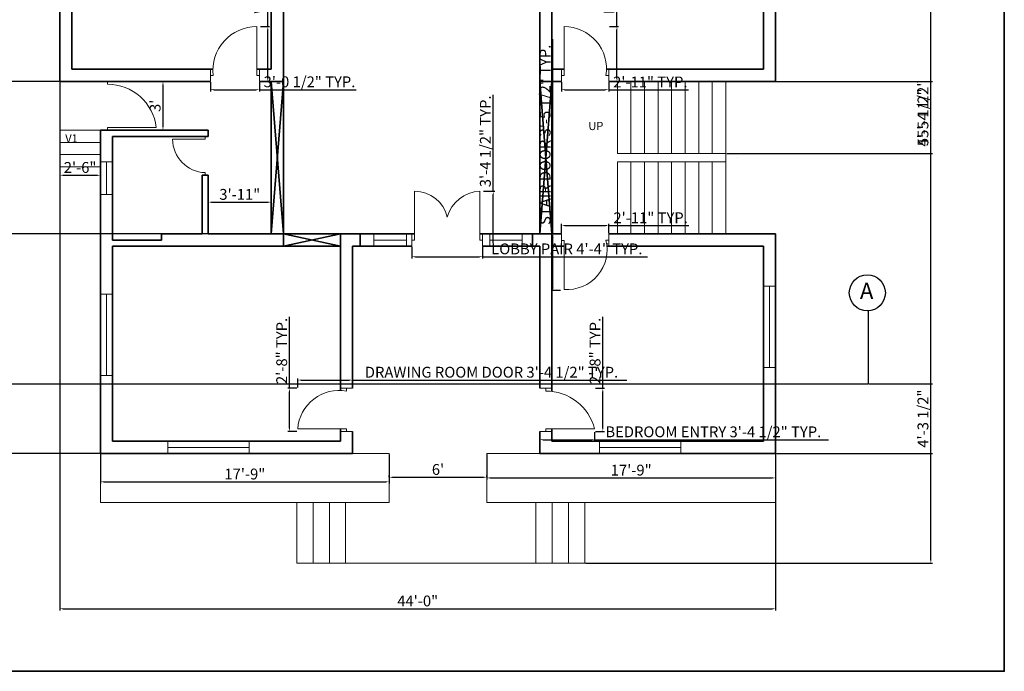
# Model space of a CAD drawing. Units: inches. Extents: x 2257 to 3678, y 834 to 1975.
# Tile 7 of 16: x 2952 to 3678, y 849 to 1330. Entities that reach past the tile are written whole.
import ezdxf

# ---------------------------------------------------------------- set-up
doc = ezdxf.new("R2010")
doc.units = ezdxf.units.IN
for name, color, linetype, lineweight in [('A-ANNO-DIMS', 2, 'Continuous', 18), ('A-ANNO-SYMB', 7, 'Continuous', 25), ('A-ANNO-TEXT', 7, 'Continuous', 18), ('A-ANNO-TTLB', 7, 'Continuous', 35), ('A-DOOR', 3, 'Continuous', 18), ('A-FLOR-STRS', 7, 'Continuous', 18), ('A-GLAZ', 4, 'Continuous', 18), ('A-WALL', 7, 'Continuous', 35)]:
    doc.layers.add(name, color=color, linetype=linetype, lineweight=lineweight)
doc.styles.get("Standard").update_dxf_attribs({"font": 'arial.ttf'})
doc.dimstyles.new('ISO-25', dxfattribs={"dimtxt": 8, "dimasz": 2.5, "dimexe": 1.25, "dimexo": 0.625, "dimtad": 1, "dimdec": 0, "dimlunit": 3, "dimtxsty": 'Standard', "dimcen": 2.5, "dimadec": 0, "dimazin": 0, "dimtfac": 1, "dimtdec": 0, "dimtmove": 0, "dimatfit": 3, "dimfxl": 1, "dimarcsym": 0})

# ---------------------------------------------------------------- blocks, each defined once
blk = doc.blocks.new('*D16')
at = {"layer": 'A-ANNO-DIMS', "color": 0, "lineweight": -2, "transparency": 16777216}
for p, q in [((3051.29, 1284.58), (3058.6, 1284.58)), ((3057.35, 1282.08), (3057.35, 1251.08)), ((3051.29, 1248.58), (3058.6, 1248.58))]:
    blk.add_line(p, q, dxfattribs=at)
at = {"layer": 'A-ANNO-DIMS', "color": 0, "transparency": 16777216}
for points in [[(3056.93, 1282.08), (3057.77, 1282.08), (3057.35, 1284.58)], [(3056.93, 1251.08), (3057.77, 1251.08), (3057.35, 1248.58)]]:
    blk.add_solid(points, dxfattribs=at)
at = {"layer": 'Defpoints', "color": 0, "transparency": 16777216}
for p in [(3050.66, 1284.58), (3050.66, 1248.58), (3057.35, 1248.58)]:
    blk.add_point(p, dxfattribs=at)
at = {"layer": 'A-ANNO-DIMS', "color": 0, "transparency": 16777216, "insert": (3052.64, 1266.58), "char_height": 8, "attachment_point": 5, "rotation": 90}
blk.add_mtext("3'", dxfattribs=at)
blk = doc.blocks.new('*D10')
at = {"layer": 'A-ANNO-DIMS', "color": 0, "lineweight": -2, "transparency": 16777216}
for p, q in [((3090.74, 1196.14), (3090.74, 1196.77)), ((3093.24, 1195.52), (3134.74, 1195.52)), ((3137.24, 1196.14), (3137.24, 1196.77))]:
    blk.add_line(p, q, dxfattribs=at)
at = {"layer": 'A-ANNO-DIMS', "color": 0, "transparency": 16777216}
for points in [[(3093.24, 1195.94), (3093.24, 1195.1), (3090.74, 1195.52)], [(3134.74, 1195.94), (3134.74, 1195.1), (3137.24, 1195.52)]]:
    blk.add_solid(points, dxfattribs=at)
at = {"layer": 'Defpoints', "color": 0, "transparency": 16777216}
for p in [(3090.74, 1195.52), (3137.24, 1195.52), (3137.24, 1195.52)]:
    blk.add_point(p, dxfattribs=at)
at = {"layer": 'A-ANNO-DIMS', "color": 0, "transparency": 16777216, "insert": (3113.99, 1200.23), "char_height": 8, "attachment_point": 5}
blk.add_mtext('3\'-11"', dxfattribs=at)
blk = doc.blocks.new('*D11')
at = {"layer": 'A-ANNO-DIMS', "color": 0, "lineweight": -2, "transparency": 16777216}
for p, q in [((2981.24, 1220.95), (2981.24, 1214.14)), ((3011.24, 1220.95), (3011.24, 1214.14)), ((2983.74, 1215.39), (3008.74, 1215.39))]:
    blk.add_line(p, q, dxfattribs=at)
at = {"layer": 'A-ANNO-DIMS', "color": 0, "transparency": 16777216}
for points in [[(2983.74, 1215.8), (2983.74, 1214.97), (2981.24, 1215.39)], [(3008.74, 1215.8), (3008.74, 1214.97), (3011.24, 1215.39)]]:
    blk.add_solid(points, dxfattribs=at)
at = {"layer": 'Defpoints', "color": 0, "transparency": 16777216}
for p in [(2981.24, 1221.58), (3011.24, 1221.58), (3011.24, 1215.39)]:
    blk.add_point(p, dxfattribs=at)
at = {"layer": 'A-ANNO-DIMS', "color": 0, "transparency": 16777216, "insert": (2996.24, 1220.09), "char_height": 8, "attachment_point": 5}
blk.add_mtext('2\'-6"', dxfattribs=at)
blk = doc.blocks.new('*D12')
at = {"layer": 'A-ANNO-DIMS', "color": 0, "lineweight": -2, "transparency": 16777216}
for p, q in [((3011.24, 1009.45), (3011.24, 987.96)), ((3224.24, 1009.45), (3224.24, 987.96)), ((3013.74, 989.21), (3221.74, 989.21))]:
    blk.add_line(p, q, dxfattribs=at)
at = {"layer": 'A-ANNO-DIMS', "color": 0, "transparency": 16777216}
for points in [[(3013.74, 989.62), (3013.74, 988.79), (3011.24, 989.21)], [(3221.74, 989.62), (3221.74, 988.79), (3224.24, 989.21)]]:
    blk.add_solid(points, dxfattribs=at)
at = {"layer": 'Defpoints', "color": 0, "transparency": 16777216}
for p in [(3011.24, 1010.08), (3224.24, 1010.08), (3224.24, 989.21)]:
    blk.add_point(p, dxfattribs=at)
at = {"layer": 'A-ANNO-DIMS', "color": 0, "transparency": 16777216, "insert": (3117.74, 993.92), "char_height": 8, "attachment_point": 5}
blk.add_mtext('17\'-9"', dxfattribs=at)
blk = doc.blocks.new('*D13')
at = {"layer": 'A-ANNO-DIMS', "color": 0, "lineweight": -2, "transparency": 16777216}
for p, q in [((3296.24, 1009.45), (3296.24, 990.83)), ((3509.24, 1009.45), (3509.24, 990.83)), ((3298.74, 992.08), (3506.74, 992.08))]:
    blk.add_line(p, q, dxfattribs=at)
at = {"layer": 'A-ANNO-DIMS', "color": 0, "transparency": 16777216}
for points in [[(3298.74, 992.49), (3298.74, 991.66), (3296.24, 992.08)], [(3506.74, 992.49), (3506.74, 991.66), (3509.24, 992.08)]]:
    blk.add_solid(points, dxfattribs=at)
at = {"layer": 'Defpoints', "color": 0, "transparency": 16777216}
for p in [(3296.24, 1010.08), (3509.24, 1010.08), (3509.24, 992.08)]:
    blk.add_point(p, dxfattribs=at)
at = {"layer": 'A-ANNO-DIMS', "color": 0, "transparency": 16777216, "insert": (3402.74, 996.79), "char_height": 8, "attachment_point": 5}
blk.add_mtext('17\'-9"', dxfattribs=at)
blk = doc.blocks.new('*D14')
at = {"layer": 'A-ANNO-DIMS', "color": 0, "lineweight": -2, "transparency": 16777216}
for p, q in [((3224.24, 992.7), (3224.24, 993.82)), ((3226.74, 992.57), (3293.74, 992.57)), ((3296.24, 992.7), (3296.24, 993.82))]:
    blk.add_line(p, q, dxfattribs=at)
at = {"layer": 'A-ANNO-DIMS', "color": 0, "transparency": 16777216}
for points in [[(3226.74, 992.99), (3226.74, 992.16), (3224.24, 992.57)], [(3293.74, 992.99), (3293.74, 992.16), (3296.24, 992.57)]]:
    blk.add_solid(points, dxfattribs=at)
at = {"layer": 'Defpoints', "color": 0, "transparency": 16777216}
for p in [(3224.24, 992.08), (3296.24, 992.57), (3296.24, 992.08)]:
    blk.add_point(p, dxfattribs=at)
at = {"layer": 'A-ANNO-DIMS', "color": 0, "transparency": 16777216, "insert": (3260.24, 997.28), "char_height": 8, "attachment_point": 5}
blk.add_mtext("6'", dxfattribs=at)
blk = doc.blocks.new('WIN-60')
for p, q in [((0, 9), (0, 0)), ((60, 4.5), (60, 9)), ((60, 9), (60, 0)), ((0, 0), (0, 4.5)), ((0, 4.5), (60, 4.5))]:
    blk.add_line(p, q)
blk = doc.blocks.new('WIN-60-SIDE')
for p, q in [((0, 60), (9, 60)), ((9, 60), (4.5, 60)), ((4.5, 60), (4.5, 0)), ((9, 0), (0, 0)), ((4.5, 0), (9, 0))]:
    blk.add_line(p, q)
blk = doc.blocks.new('WIN-24')
for p, q in [((0, 9), (0, 0)), ((24, 4.5), (24, 9)), ((24, 9), (24, 0)), ((0, 0), (0, 4.5)), ((0, 4.5), (24, 4.5))]:
    blk.add_line(p, q)
blk = doc.blocks.new('DOOR-WC')
for p, q in [((24, 26.75), (0, 26.75)), ((24, 28.75), (24, 26.75)), ((24, 26.75), (24, 28.75)), ((24, 0), (24, 2)), ((24, 0), (24, 2))]:
    blk.add_line(p, q)
blk.add_arc((24.77, 26.75), 24.77, 180, 268.22548)
blk = doc.blocks.new('DOOR-BEDROOM-WEST')
for p, q in [((34.29, 4.5), (34.29, 40.5)), ((0, 9), (0, 0)), ((36.29, 9), (36.29, 0)), ((0, 0), (0, 4.5)), ((0, 4.5), (2, 4.5)), ((36.29, 4.5), (34.29, 4.5)), ((36.29, 0), (36.29, 4.5)), ((0, 0), (0, 0))]:
    blk.add_line(p, q)
blk.add_arc((34.29, 8.02), 32.48, 90, 186.22352)
blk = doc.blocks.new('DOOR-LOBBY-PAIR')
for p, q in [((2, 4.5), (2, 40.5)), ((50.14, 4.5), (50.14, 40.5)), ((0, 0), (0, 9)), ((0, 9), (0, 4.5)), ((52.14, 9), (52.14, 0)), ((0, 4.5), (2, 4.5)), ((52.14, 4.5), (50.14, 4.5)), ((52.14, 0), (52.14, 4.5))]:
    blk.add_line(p, q)
for centre, radius, start, end in [((2, 15.75), 24.75, 13.39446, 90), ((50.98, 14.71), 25.8, 91.86682, 164.78752)]:
    blk.add_arc(centre, radius, start, end)
blk = doc.blocks.new('DOOR-BEDROOM-EAST')
for p, q in [((2, 4.5), (2, 40.5)), ((0, 9), (0, 0)), ((34.84, 0), (34.84, 9)), ((34.84, 9), (34.84, 4.5)), ((0, 4.5), (2, 4.5)), ((34.84, 4.5), (32.84, 4.5))]:
    blk.add_line(p, q)
blk.add_arc((2, 9.29), 31.21, 351.16993, 90)
blk = doc.blocks.new('DOOR-BEDROOM-FRONT')
for p, q in [((0, 41.01), (0, 32.01)), ((34.84, 36.51), (32.84, 36.51)), ((34.84, 41.01), (34.84, 32.01)), ((34.84, 32.01), (34.84, 36.51)), ((0, 36.08), (2, 36.08)), ((2, 36.08), (2, 0.08))]:
    blk.add_line(p, q)
blk.add_arc((4.15, 29.52), 29.53, 265.82197, 13.68707)
blk = doc.blocks.new('DOOR-DRAWING-ROOM')
for p, q in [((31.5, 31.83), (40.5, 31.83)), ((40.5, 31.83), (36, 31.83)), ((36, 31.83), (36, 29.83)), ((36, 2), (0, 2)), ((36, 0), (36, 2)), ((31.5, 0), (40.5, 0)), ((40.5, 0), (36, 0))]:
    blk.add_line(p, q)
blk.add_arc((30.7, -0.52), 30.81, 80.10035, 175.31629)
blk = doc.blocks.new('DOOR-LOBBY-BEDROOM')
for p, q in [((0, 31.83), (9, 31.83)), ((9, 31.83), (4.5, 31.83)), ((4.5, 31.83), (4.5, 29.83)), ((4.5, 0), (4.5, 2)), ((4.5, 2), (40.5, 2)), ((0, 0), (0, 0)), ((0, 0), (9, 0)), ((9, 0), (4.5, 0))]:
    blk.add_line(p, q)
blk.add_arc((4.5, -7.37), 37.2, 14.58337, 90)
blk = doc.blocks.new('DOOR-SIDE-ENTRY')
for p, q in [((0, 36), (0, 34)), ((0, 0), (0, 2)), ((0, 2), (24, 2)), ((24, 2), (36, 2))]:
    blk.add_line(p, q)
blk.add_arc((0, -2.25), 36.25, 6.73292, 90)
blk = doc.blocks.new('STEPS-VERANDAH')
for p, q in [((0, 80.97), (213, 80.97)), ((0, 44.97), (0, 80.97)), ((0, 80.97), (0, 80.97)), ((213, 80.97), (213, 44.97)), ((213, 80.97), (213, 44.97)), ((498, 80.97), (285, 80.97)), ((285, 80.97), (285, 44.97)), ((285, 80.97), (285, 44.97)), ((498, 44.97), (498, 80.97)), ((213, 44.97), (0, 44.97)), ((144.84, 0), (144.84, 44.97)), ((168.84, 44.97), (156.84, 44.97)), ((156.84, 44.97), (156.84, 0)), ((168.84, 0), (168.84, 44.97)), ((168.84, 44.97), (168.84, 44.97)), ((180.84, 44.97), (180.84, 0)), ((285, 44.97), (498, 44.97)), ((333.2, 44.97), (321.2, 44.97)), ((321.2, 44.97), (321.2, 0)), ((333.2, 0), (333.2, 44.97)), ((357.2, 44.97), (345.2, 44.97)), ((345.2, 44.97), (345.2, 0)), ((357.2, 0), (357.2, 44.97)), ((213, 0), (144.84, 0)), ((156.84, 0), (144.84, 0)), ((180.84, 0), (168.84, 0)), ((213, 0), (357.2, 0)), ((345.2, 0), (333.2, 0))]:
    blk.add_line(p, q)
blk = doc.blocks.new('STEPS-SIDE-ENTRY')
for p, q in [((0, 69.18), (0, 3.09)), ((30, 30.09), (0, 30.09)), ((30, 18), (30, 27)), ((0, 12.09), (0, 21.09)), ((0, 21.09), (30, 21.09)), ((30, 12.09), (0, 12.09)), ((30, 0), (30, 9)), ((0, 3.09), (30, 3.09))]:
    blk.add_line(p, q)
blk = doc.blocks.new('*D64')
at = {"layer": 'A-ANNO-DIMS', "color": 0, "lineweight": -2, "transparency": 16777216}
for p, q in [((3134.67, 1325.08), (3134.67, 1529.43)), ((3129.22, 1325.08), (3135.92, 1325.08)), ((3134.67, 1287.08), (3134.67, 1322.58)), ((3129.22, 1284.58), (3135.92, 1284.58))]:
    blk.add_line(p, q, dxfattribs=at)
at = {"layer": 'A-ANNO-DIMS', "color": 0, "transparency": 16777216}
for points in [[(3134.25, 1322.58), (3135.09, 1322.58), (3134.67, 1325.08)], [(3134.25, 1287.08), (3135.09, 1287.08), (3134.67, 1284.58)]]:
    blk.add_solid(points, dxfattribs=at)
at = {"layer": 'Defpoints', "color": 0, "transparency": 16777216}
for p in [(3128.6, 1325.08), (3134.67, 1325.08), (3128.6, 1284.58)]:
    blk.add_point(p, dxfattribs=at)
at = {"layer": 'A-ANNO-DIMS', "color": 0, "transparency": 16777216, "insert": (3129.9, 1428.5), "char_height": 8, "attachment_point": 5, "rotation": 90}
blk.add_mtext('WEST BEDROOM DOOR 3\'-4 1/2" TYP.', dxfattribs=at)
blk = doc.blocks.new('*D65')
at = {"layer": 'A-ANNO-DIMS', "color": 0, "lineweight": -2, "transparency": 16777216}
for p, q in [((3092.31, 1283.95), (3092.31, 1277.25)), ((3094.81, 1278.5), (3126.1, 1278.5)), ((3128.6, 1283.95), (3128.6, 1277.25)), ((3128.6, 1278.5), (3199.75, 1278.5))]:
    blk.add_line(p, q, dxfattribs=at)
at = {"layer": 'A-ANNO-DIMS', "color": 0, "transparency": 16777216}
for points in [[(3094.81, 1278.92), (3094.81, 1278.09), (3092.31, 1278.5)], [(3126.1, 1278.92), (3126.1, 1278.09), (3128.6, 1278.5)]]:
    blk.add_solid(points, dxfattribs=at)
at = {"layer": 'Defpoints', "color": 0, "transparency": 16777216}
for p in [(3092.31, 1284.58), (3128.6, 1284.58), (3128.6, 1278.5)]:
    blk.add_point(p, dxfattribs=at)
at = {"layer": 'A-ANNO-DIMS', "color": 0, "transparency": 16777216, "insert": (3165.42, 1283.27), "char_height": 8, "attachment_point": 5}
blk.add_mtext('3\'-0 1/2" TYP.', dxfattribs=at)
blk = doc.blocks.new('*D66')
at = {"layer": 'A-ANNO-DIMS', "color": 0, "lineweight": -2, "transparency": 16777216}
for p, q in [((3392.2, 1325.08), (3392.2, 1525.59)), ((3386.75, 1325.08), (3393.45, 1325.08)), ((3392.2, 1287.08), (3392.2, 1322.58)), ((3386.75, 1284.58), (3393.45, 1284.58))]:
    blk.add_line(p, q, dxfattribs=at)
at = {"layer": 'A-ANNO-DIMS', "color": 0, "transparency": 16777216}
for points in [[(3391.79, 1322.58), (3392.62, 1322.58), (3392.2, 1325.08)], [(3391.79, 1287.08), (3392.62, 1287.08), (3392.2, 1284.58)]]:
    blk.add_solid(points, dxfattribs=at)
at = {"layer": 'Defpoints', "color": 0, "transparency": 16777216}
for p in [(3386.13, 1325.08), (3392.2, 1325.08), (3386.13, 1284.58)]:
    blk.add_point(p, dxfattribs=at)
at = {"layer": 'A-ANNO-DIMS', "color": 0, "transparency": 16777216, "insert": (3387.44, 1426.58), "char_height": 8, "attachment_point": 5, "rotation": 90}
blk.add_mtext('EAST BEDROOM DOOR 3\'-4 1/2" TYP.', dxfattribs=at)
blk = doc.blocks.new('*D67')
at = {"layer": 'A-ANNO-DIMS', "color": 0, "lineweight": -2, "transparency": 16777216}
for p, q in [((3351.29, 1283.95), (3351.29, 1277.25)), ((3353.79, 1278.5), (3383.63, 1278.5)), ((3386.13, 1283.95), (3386.13, 1277.25)), ((3386.13, 1278.5), (3445, 1278.5))]:
    blk.add_line(p, q, dxfattribs=at)
at = {"layer": 'A-ANNO-DIMS', "color": 0, "transparency": 16777216}
for points in [[(3353.79, 1278.92), (3353.79, 1278.09), (3351.29, 1278.5)], [(3383.63, 1278.92), (3383.63, 1278.09), (3386.13, 1278.5)]]:
    blk.add_solid(points, dxfattribs=at)
at = {"layer": 'Defpoints', "color": 0, "transparency": 16777216}
for p in [(3351.29, 1284.58), (3386.13, 1284.58), (3386.13, 1278.5)]:
    blk.add_point(p, dxfattribs=at)
at = {"layer": 'A-ANNO-DIMS', "color": 0, "transparency": 16777216, "insert": (3416.81, 1283.15), "char_height": 8, "attachment_point": 5}
blk.add_mtext('2\'-11" TYP.', dxfattribs=at)
blk = doc.blocks.new('*D68')
at = {"layer": 'A-ANNO-DIMS', "color": 0, "lineweight": -2, "transparency": 16777216}
for p, q in [((3345.05, 1172.08), (3345.05, 1315.84)), ((3350.66, 1172.08), (3343.8, 1172.08)), ((3345.05, 1132.95), (3345.05, 1169.58)), ((3350.66, 1130.45), (3343.8, 1130.45))]:
    blk.add_line(p, q, dxfattribs=at)
at = {"layer": 'A-ANNO-DIMS', "color": 0, "transparency": 16777216}
for points in [[(3344.63, 1169.58), (3345.46, 1169.58), (3345.05, 1172.08)], [(3344.63, 1132.95), (3345.46, 1132.95), (3345.05, 1130.45)]]:
    blk.add_solid(points, dxfattribs=at)
at = {"layer": 'Defpoints', "color": 0, "transparency": 16777216}
for p in [(3345.05, 1172.08), (3351.29, 1172.08), (3351.29, 1130.45)]:
    blk.add_point(p, dxfattribs=at)
at = {"layer": 'A-ANNO-DIMS', "color": 0, "transparency": 16777216, "insert": (3340.28, 1245.21), "char_height": 8, "attachment_point": 5, "rotation": 90}
blk.add_mtext('STAIR DOOR 3\'-5 1/2" TYP.', dxfattribs=at)
blk = doc.blocks.new('*D69')
at = {"layer": 'A-ANNO-DIMS', "color": 0, "lineweight": -2, "transparency": 16777216}
for p, q in [((3351.29, 1172.7), (3351.29, 1179.57)), ((3353.79, 1178.32), (3383.86, 1178.32)), ((3386.36, 1172.7), (3386.36, 1179.57)), ((3386.36, 1178.32), (3445.23, 1178.32))]:
    blk.add_line(p, q, dxfattribs=at)
at = {"layer": 'A-ANNO-DIMS', "color": 0, "transparency": 16777216}
for points in [[(3353.79, 1178.74), (3353.79, 1177.9), (3351.29, 1178.32)], [(3383.86, 1178.74), (3383.86, 1177.9), (3386.36, 1178.32)]]:
    blk.add_solid(points, dxfattribs=at)
at = {"layer": 'Defpoints', "color": 0, "transparency": 16777216}
for p in [(3386.36, 1178.32), (3351.29, 1172.08), (3386.36, 1172.08)]:
    blk.add_point(p, dxfattribs=at)
at = {"layer": 'A-ANNO-DIMS', "color": 0, "transparency": 16777216, "insert": (3417.05, 1182.96), "char_height": 8, "attachment_point": 5}
blk.add_mtext('2\'-11" TYP.', dxfattribs=at)
blk = doc.blocks.new('*D74')
at = {"layer": 'A-ANNO-DIMS', "color": 0, "lineweight": -2, "transparency": 16777216}
for p, q in [((3241.01, 1162.45), (3241.01, 1154.01)), ((3293.15, 1162.45), (3293.15, 1154.01)), ((3243.51, 1155.26), (3290.65, 1155.26)), ((3293.15, 1155.26), (3414.87, 1155.26))]:
    blk.add_line(p, q, dxfattribs=at)
at = {"layer": 'A-ANNO-DIMS', "color": 0, "transparency": 16777216}
for points in [[(3243.51, 1155.67), (3243.51, 1154.84), (3241.01, 1155.26)], [(3290.65, 1155.67), (3290.65, 1154.84), (3293.15, 1155.26)]]:
    blk.add_solid(points, dxfattribs=at)
at = {"layer": 'Defpoints', "color": 0, "transparency": 16777216}
for p in [(3241.01, 1163.08), (3293.15, 1163.08), (3293.15, 1155.26)]:
    blk.add_point(p, dxfattribs=at)
at = {"layer": 'A-ANNO-DIMS', "color": 0, "transparency": 16777216, "insert": (3355.26, 1160.02), "char_height": 8, "attachment_point": 5}
blk.add_mtext('LOBBY PAIR 4\'-4" TYP.', dxfattribs=at)
blk = doc.blocks.new('*D75')
at = {"layer": 'A-ANNO-DIMS', "color": 0, "lineweight": -2, "transparency": 16777216}
for p, q in [((3300.97, 1203.58), (3300.97, 1274.73)), ((3293.77, 1203.58), (3302.22, 1203.58)), ((3300.97, 1165.58), (3300.97, 1201.08)), ((3293.77, 1163.08), (3302.22, 1163.08))]:
    blk.add_line(p, q, dxfattribs=at)
at = {"layer": 'A-ANNO-DIMS', "color": 0, "transparency": 16777216}
for points in [[(3300.55, 1201.08), (3301.38, 1201.08), (3300.97, 1203.58)], [(3300.55, 1165.58), (3301.38, 1165.58), (3300.97, 1163.08)]]:
    blk.add_solid(points, dxfattribs=at)
at = {"layer": 'Defpoints', "color": 0, "transparency": 16777216}
for p in [(3293.15, 1203.58), (3300.97, 1203.58), (3293.15, 1163.08)]:
    blk.add_point(p, dxfattribs=at)
at = {"layer": 'A-ANNO-DIMS', "color": 0, "transparency": 16777216, "insert": (3296.2, 1240.4), "char_height": 8, "attachment_point": 5, "rotation": 90}
blk.add_mtext('3\'-4 1/2" TYP.', dxfattribs=at)
blk = doc.blocks.new('*D76')
at = {"layer": 'A-ANNO-DIMS', "color": 0, "lineweight": -2, "transparency": 16777216}
for p, q in [((3156.74, 1058.81), (3156.74, 1065.51)), ((3159.24, 1064.26), (3194.74, 1064.26)), ((3197.24, 1058.81), (3197.24, 1065.51)), ((3197.24, 1064.26), (3399.62, 1064.26))]:
    blk.add_line(p, q, dxfattribs=at)
at = {"layer": 'A-ANNO-DIMS', "color": 0, "transparency": 16777216}
for points in [[(3159.24, 1064.68), (3159.24, 1063.85), (3156.74, 1064.26)], [(3194.74, 1064.68), (3194.74, 1063.85), (3197.24, 1064.26)]]:
    blk.add_solid(points, dxfattribs=at)
at = {"layer": 'Defpoints', "color": 0, "transparency": 16777216}
for p in [(3197.24, 1064.26), (3156.74, 1058.19), (3197.24, 1058.19)]:
    blk.add_point(p, dxfattribs=at)
at = {"layer": 'A-ANNO-DIMS', "color": 0, "transparency": 16777216, "insert": (3299.68, 1069.03), "char_height": 8, "attachment_point": 5}
blk.add_mtext('DRAWING ROOM DOOR 3\'-4 1/2" TYP.', dxfattribs=at)
blk = doc.blocks.new('*D77')
at = {"layer": 'A-ANNO-DIMS', "color": 0, "lineweight": -2, "transparency": 16777216}
for p, q in [((3150.67, 1058.19), (3150.67, 1110.84)), ((3156.12, 1058.19), (3149.42, 1058.19)), ((3150.67, 1028.85), (3150.67, 1055.69)), ((3156.12, 1026.35), (3149.42, 1026.35))]:
    blk.add_line(p, q, dxfattribs=at)
at = {"layer": 'A-ANNO-DIMS', "color": 0, "transparency": 16777216}
for points in [[(3150.25, 1055.69), (3151.08, 1055.69), (3150.67, 1058.19)], [(3150.25, 1028.85), (3151.08, 1028.85), (3150.67, 1026.35)]]:
    blk.add_solid(points, dxfattribs=at)
at = {"layer": 'Defpoints', "color": 0, "transparency": 16777216}
for p in [(3150.67, 1058.19), (3156.74, 1058.19), (3156.74, 1026.35)]:
    blk.add_point(p, dxfattribs=at)
at = {"layer": 'A-ANNO-DIMS', "color": 0, "transparency": 16777216, "insert": (3145.96, 1085.76), "char_height": 8, "attachment_point": 5, "rotation": 90}
blk.add_mtext('2\'-8" TYP.', dxfattribs=at)
blk = doc.blocks.new('*D78')
at = {"layer": 'A-ANNO-DIMS', "color": 0, "lineweight": -2, "transparency": 16777216}
for p, q in [((3335.24, 1025.73), (3335.24, 1019.03)), ((3375.74, 1025.73), (3375.74, 1019.03)), ((3337.74, 1020.28), (3373.24, 1020.28)), ((3375.74, 1020.28), (3548.37, 1020.28))]:
    blk.add_line(p, q, dxfattribs=at)
at = {"layer": 'A-ANNO-DIMS', "color": 0, "transparency": 16777216}
for points in [[(3337.74, 1020.7), (3337.74, 1019.86), (3335.24, 1020.28)], [(3373.24, 1020.7), (3373.24, 1019.86), (3375.74, 1020.28)]]:
    blk.add_solid(points, dxfattribs=at)
at = {"layer": 'Defpoints', "color": 0, "transparency": 16777216}
for p in [(3335.24, 1026.35), (3375.74, 1026.35), (3375.74, 1020.28)]:
    blk.add_point(p, dxfattribs=at)
at = {"layer": 'A-ANNO-DIMS', "color": 0, "transparency": 16777216, "insert": (3463.31, 1025.05), "char_height": 8, "attachment_point": 5}
blk.add_mtext('BEDROOM ENTRY 3\'-4 1/2" TYP.', dxfattribs=at)
blk = doc.blocks.new('*D79')
at = {"layer": 'A-ANNO-DIMS', "color": 0, "lineweight": -2, "transparency": 16777216}
for p, q in [((3381.82, 1058.19), (3381.82, 1110.84)), ((3376.37, 1058.19), (3383.07, 1058.19)), ((3381.82, 1028.85), (3381.82, 1055.69)), ((3376.37, 1026.35), (3383.07, 1026.35))]:
    blk.add_line(p, q, dxfattribs=at)
at = {"layer": 'A-ANNO-DIMS', "color": 0, "transparency": 16777216}
for points in [[(3381.4, 1055.69), (3382.23, 1055.69), (3381.82, 1058.19)], [(3381.4, 1028.85), (3382.23, 1028.85), (3381.82, 1026.35)]]:
    blk.add_solid(points, dxfattribs=at)
at = {"layer": 'Defpoints', "color": 0, "transparency": 16777216}
for p in [(3375.74, 1058.19), (3381.82, 1058.19), (3375.74, 1026.35)]:
    blk.add_point(p, dxfattribs=at)
at = {"layer": 'A-ANNO-DIMS', "color": 0, "transparency": 16777216, "insert": (3377.11, 1085.76), "char_height": 8, "attachment_point": 5, "rotation": 90}
blk.add_mtext('2\'-8" TYP.', dxfattribs=at)
blk = doc.blocks.new('*D99')
at = {"layer": 'A-ANNO-DIMS', "color": 0, "lineweight": -2, "transparency": 16777216}
for p, q in [((2981.24, 1283.95), (2981.24, 894.3)), ((3509.24, 1009.45), (3509.24, 894.3)), ((2983.74, 895.55), (3506.74, 895.55))]:
    blk.add_line(p, q, dxfattribs=at)
at = {"layer": 'A-ANNO-DIMS', "color": 0, "transparency": 16777216}
for points in [[(2983.74, 895.97), (2983.74, 895.14), (2981.24, 895.55)], [(3506.74, 895.97), (3506.74, 895.14), (3509.24, 895.55)]]:
    blk.add_solid(points, dxfattribs=at)
at = {"layer": 'Defpoints', "color": 0, "transparency": 16777216}
for p in [(2981.24, 1284.58), (3509.24, 1010.08), (3509.24, 895.55)]:
    blk.add_point(p, dxfattribs=at)
at = {"layer": 'A-ANNO-DIMS', "color": 0, "transparency": 16777216, "insert": (3245.24, 900.26), "char_height": 8, "attachment_point": 5}
blk.add_mtext('44\'-0"', dxfattribs=at)
blk = doc.blocks.new('*D100')
at = {"layer": 'A-ANNO-DIMS', "color": 0, "lineweight": -2, "transparency": 16777216}
for p, q in [((3479.87, 1593.58), (3625.01, 1593.58)), ((3623.76, 931.6), (3623.76, 1591.08)), ((3369.06, 929.1), (3625.01, 929.1))]:
    blk.add_line(p, q, dxfattribs=at)
at = {"layer": 'A-ANNO-DIMS', "color": 0, "transparency": 16777216}
for points in [[(3623.34, 1591.08), (3624.17, 1591.08), (3623.76, 1593.58)], [(3623.34, 931.6), (3624.17, 931.6), (3623.76, 929.1)]]:
    blk.add_solid(points, dxfattribs=at)
at = {"layer": 'Defpoints', "color": 0, "transparency": 16777216}
for p in [(3479.24, 1593.58), (3623.76, 1593.58), (3368.44, 929.1)]:
    blk.add_point(p, dxfattribs=at)
at = {"layer": 'A-ANNO-DIMS', "color": 0, "transparency": 16777216, "insert": (3618.99, 1261.34), "char_height": 8, "attachment_point": 5, "rotation": 90}
blk.add_mtext('55\'-4 1/2"', dxfattribs=at)
blk = doc.blocks.new('*D101')
at = {"layer": 'A-ANNO-DIMS', "color": 0, "lineweight": -2, "transparency": 16777216}
for p, q in [((3136.62, 1172.08), (2896.72, 1172.08)), ((2897.97, 1012.58), (2897.97, 1169.58)), ((3010.62, 1010.08), (2896.72, 1010.08))]:
    blk.add_line(p, q, dxfattribs=at)
at = {"layer": 'A-ANNO-DIMS', "color": 0, "transparency": 16777216}
for points in [[(2897.55, 1169.58), (2898.38, 1169.58), (2897.97, 1172.08)], [(2897.55, 1012.58), (2898.38, 1012.58), (2897.97, 1010.08)]]:
    blk.add_solid(points, dxfattribs=at)
at = {"layer": 'Defpoints', "color": 0, "transparency": 16777216}
for p in [(2897.97, 1172.08), (3137.24, 1172.08), (3011.24, 1010.08)]:
    blk.add_point(p, dxfattribs=at)
at = {"layer": 'A-ANNO-DIMS', "color": 0, "transparency": 16777216, "insert": (2893.25, 1091.08), "char_height": 8, "attachment_point": 5, "rotation": 90}
blk.add_mtext('13\'-6"', dxfattribs=at)
blk = doc.blocks.new('*D102')
at = {"layer": 'A-ANNO-DIMS', "color": 0, "lineweight": -2, "transparency": 16777216}
for p, q in [((2980.62, 1284.58), (2896.72, 1284.58)), ((2897.97, 1174.58), (2897.97, 1282.08)), ((3136.62, 1172.08), (2896.72, 1172.08))]:
    blk.add_line(p, q, dxfattribs=at)
at = {"layer": 'A-ANNO-DIMS', "color": 0, "transparency": 16777216}
for points in [[(2897.55, 1282.08), (2898.38, 1282.08), (2897.97, 1284.58)], [(2897.55, 1174.58), (2898.38, 1174.58), (2897.97, 1172.08)]]:
    blk.add_solid(points, dxfattribs=at)
at = {"layer": 'Defpoints', "color": 0, "transparency": 16777216}
for p in [(2897.97, 1284.58), (2981.24, 1284.58), (3137.24, 1172.08)]:
    blk.add_point(p, dxfattribs=at)
at = {"layer": 'A-ANNO-DIMS', "color": 0, "transparency": 16777216, "insert": (2893.21, 1228.33), "char_height": 8, "attachment_point": 5, "rotation": 90}
blk.add_mtext('9\'-4 1/2"', dxfattribs=at)
blk = doc.blocks.new('*D103')
at = {"layer": 'A-ANNO-DIMS', "color": 0, "lineweight": -2, "transparency": 16777216}
for p, q in [((2980.62, 1440.58), (2896.72, 1440.58)), ((2897.97, 1287.08), (2897.97, 1438.08)), ((2980.62, 1284.58), (2896.72, 1284.58))]:
    blk.add_line(p, q, dxfattribs=at)
at = {"layer": 'A-ANNO-DIMS', "color": 0, "transparency": 16777216}
for points in [[(2897.55, 1438.08), (2898.38, 1438.08), (2897.97, 1440.58)], [(2897.55, 1287.08), (2898.38, 1287.08), (2897.97, 1284.58)]]:
    blk.add_solid(points, dxfattribs=at)
at = {"layer": 'Defpoints', "color": 0, "transparency": 16777216}
for p in [(2897.97, 1440.58), (2981.24, 1440.58), (2981.24, 1284.58)]:
    blk.add_point(p, dxfattribs=at)
at = {"layer": 'A-ANNO-DIMS', "color": 0, "transparency": 16777216, "insert": (2893.25, 1362.58), "char_height": 8, "attachment_point": 5, "rotation": 90}
blk.add_mtext('13\'-0"', dxfattribs=at)
blk = doc.blocks.new('*D105')
at = {"layer": 'A-ANNO-DIMS', "color": 0, "lineweight": -2, "transparency": 16777216}
for p, q in [((3578.29, 1061.57), (3625.01, 1061.57)), ((3623.76, 1012.58), (3623.76, 1059.07)), ((3509.87, 1010.08), (3625.01, 1010.08))]:
    blk.add_line(p, q, dxfattribs=at)
at = {"layer": 'A-ANNO-DIMS', "color": 0, "transparency": 16777216}
for points in [[(3623.34, 1059.07), (3624.17, 1059.07), (3623.76, 1061.57)], [(3623.34, 1012.58), (3624.17, 1012.58), (3623.76, 1010.08)]]:
    blk.add_solid(points, dxfattribs=at)
at = {"layer": 'Defpoints', "color": 0, "transparency": 16777216}
for p in [(3577.66, 1061.57), (3623.76, 1061.57), (3509.24, 1010.08)]:
    blk.add_point(p, dxfattribs=at)
at = {"layer": 'A-ANNO-DIMS', "color": 0, "transparency": 16777216, "insert": (3618.99, 1035.83), "char_height": 8, "attachment_point": 5, "rotation": 90}
blk.add_mtext('4\'-3 1/2"', dxfattribs=at)
blk = doc.blocks.new('*D114')
at = {"layer": 'A-ANNO-DIMS', "color": 0, "lineweight": -2, "transparency": 16777216}
for p, q in [((3473.16, 1284.58), (3625.01, 1284.58)), ((3623.76, 1233.83), (3623.76, 1282.08)), ((3473.16, 1231.33), (3625.01, 1231.33))]:
    blk.add_line(p, q, dxfattribs=at)
at = {"layer": 'A-ANNO-DIMS', "color": 0, "transparency": 16777216}
for points in [[(3623.34, 1282.08), (3624.17, 1282.08), (3623.76, 1284.58)], [(3623.34, 1233.83), (3624.17, 1233.83), (3623.76, 1231.33)]]:
    blk.add_solid(points, dxfattribs=at)
at = {"layer": 'Defpoints', "color": 0, "transparency": 16777216}
for p in [(3472.54, 1284.58), (3623.76, 1284.58), (3472.54, 1231.33)]:
    blk.add_point(p, dxfattribs=at)
at = {"layer": 'A-ANNO-DIMS', "color": 0, "transparency": 16777216, "insert": (3618.99, 1257.95), "char_height": 8, "attachment_point": 5, "rotation": 90}
blk.add_mtext('4\'-5 1/2"', dxfattribs=at)

msp = doc.modelspace()

# ---------------------------------------------------------------- linework, layer by layer
at = {"layer": 'A-ANNO-SYMB'}
for p, q in [((3577.66, 1061.57), (3577.66, 1115.36)), ((2931.52, 1061.57), (3577.66, 1061.57))]:
    msp.add_line(p, q, dxfattribs=at)
msp.add_circle((3576.92, 1128.63), 13.29, dxfattribs=at)
at = {"layer": 'A-ANNO-TTLB'}
msp.add_lwpolyline([(2257.38, 1974.9), (3677.96, 1974.9), (3677.96, 849.42), (2257.38, 849.42)], close=True, dxfattribs=at)
at = {"layer": 'A-FLOR-STRS'}
for p, q in [((3392.54, 1284.58), (3392.54, 1231.33)), ((3402.54, 1284.58), (3402.54, 1231.33)), ((3412.54, 1284.58), (3412.54, 1231.33)), ((3422.54, 1284.58), (3422.54, 1231.33)), ((3432.54, 1284.58), (3432.54, 1231.33)), ((3442.54, 1284.58), (3442.54, 1231.33)), ((3452.54, 1284.58), (3452.54, 1231.33)), ((3462.54, 1284.58), (3462.54, 1231.33)), ((3472.54, 1284.58), (3472.54, 1231.33)), ((3472.54, 1231.33), (3392.54, 1231.33)), ((3472.54, 1231.33), (3472.54, 1228.01)), ((3472.54, 1228.01), (3472.54, 1225.33)), ((3481.48, 1228.33), (3481.48, 1228.33)), ((3392.54, 1225.33), (3392.54, 1172.08)), ((3392.54, 1225.33), (3472.54, 1225.33)), ((3402.54, 1225.33), (3402.54, 1172.08)), ((3412.54, 1225.33), (3412.54, 1172.08)), ((3422.54, 1225.33), (3422.54, 1172.08)), ((3432.54, 1225.33), (3432.54, 1172.08)), ((3442.54, 1225.33), (3442.54, 1172.08)), ((3452.54, 1225.33), (3452.54, 1172.08)), ((3462.54, 1225.33), (3462.54, 1172.08)), ((3472.54, 1225.33), (3472.54, 1172.08))]:
    msp.add_line(p, q, dxfattribs=at)
at = {"layer": 'A-GLAZ'}
for p, q in [((3011.24, 1225.28), (3011.24, 1225.28)), ((3212.99, 1163.08), (3212.99, 1163.08)), ((3060.99, 1014.58), (3060.99, 1014.58))]:
    msp.add_line(p, q, dxfattribs=at)
at = {"layer": 'A-WALL'}
for p, q in [((2981.24, 1440.58), (2981.24, 1284.58)), ((2990.24, 1431.58), (2990.24, 1293.58)), ((3137.24, 1431.58), (3137.24, 1293.58)), ((3146.24, 1431.58), (3146.24, 1172.08)), ((3335.24, 1431.58), (3335.24, 1172.08)), ((3335.24, 1431.58), (3335.24, 1172.08)), ((3344.24, 1431.58), (3344.24, 1172.08)), ((3500.24, 1431.58), (3500.24, 1293.58)), ((3509.24, 1431.58), (3509.24, 1284.58)), ((2990.24, 1293.58), (3094.13, 1293.58)), ((3126.6, 1293.58), (3137.24, 1293.58)), ((3344.24, 1293.58), (3353.29, 1293.58)), ((3384.5, 1293.58), (3500.24, 1293.58)), ((2981.24, 1284.58), (3092.31, 1284.58)), ((3128.6, 1284.58), (3146.24, 1284.58)), ((3137.24, 1284.58), (3137.24, 1172.08)), ((3137.24, 1284.58), (3146.24, 1172.08)), ((3137.24, 1172.08), (3146.24, 1284.58)), ((3344.24, 1284.58), (3335.24, 1284.58)), ((3344.24, 1172.08), (3335.24, 1284.58)), ((3335.24, 1284.58), (3344.24, 1284.58)), ((3344.24, 1284.58), (3335.24, 1172.08)), ((3344.24, 1284.58), (3351.29, 1284.58)), ((3386.13, 1284.58), (3509.24, 1284.58)), ((3011.24, 1248.58), (3090.74, 1248.58)), ((3011.24, 1172.08), (3011.24, 1248.58)), ((3020.24, 1244.08), (3090.74, 1244.08)), ((3020.24, 1172.08), (3020.24, 1244.08)), ((3090.74, 1244.08), (3090.74, 1248.58)), ((3086.24, 1195.52), (3086.24, 1215.32)), ((3086.24, 1215.32), (3090.74, 1215.32)), ((3090.74, 1215.32), (3090.74, 1195.52)), ((3086.24, 1172.08), (3086.24, 1195.52)), ((3090.74, 1195.52), (3090.74, 1172.08)), ((3011.24, 1172.08), (3011.24, 1010.08)), ((3020.24, 1172.08), (3020.24, 1167.58)), ((3056.24, 1172.08), (3086.24, 1172.08)), ((3056.24, 1167.58), (3056.24, 1172.08)), ((3090.74, 1172.08), (3243.01, 1172.08)), ((3146.24, 1172.08), (3146.24, 1163.08)), ((3146.24, 1163.08), (3188.24, 1172.08)), ((3188.24, 1163.08), (3146.24, 1172.08)), ((3188.24, 1172.08), (3188.24, 1056.64)), ((3188.24, 1172.08), (3188.24, 1163.08)), ((3202.85, 1172.08), (3202.85, 1163.08)), ((3291.15, 1172.08), (3335.24, 1172.08)), ((3329.89, 1172.08), (3329.89, 1172.08)), ((3329.89, 1172.08), (3329.89, 1163.08)), ((3335.24, 1172.08), (3344.24, 1172.08)), ((3344.24, 1172.08), (3351.29, 1172.08)), ((3344.24, 1172.08), (3344.24, 1163.08)), ((3344.24, 1172.08), (3344.24, 1172.08)), ((3386.13, 1172.08), (3500.24, 1172.08)), ((3500.24, 1172.08), (3509.24, 1172.08)), ((3509.24, 1172.08), (3509.24, 1010.08)), ((3011.24, 1163.08), (3011.24, 1019.08)), ((3020.24, 1167.58), (3056.24, 1167.58)), ((3020.24, 1163.08), (3188.24, 1163.08)), ((3020.24, 1163.08), (3020.24, 1019.08)), ((3090.74, 1163.08), (3086.24, 1163.08)), ((3197.24, 1163.08), (3241.01, 1163.08)), ((3197.24, 1163.08), (3197.24, 1058.19)), ((3293.15, 1163.08), (3335.24, 1163.08)), ((3335.24, 1163.08), (3335.24, 1058.19)), ((3344.24, 1163.08), (3344.24, 1055.91)), ((3344.24, 1163.08), (3353.29, 1163.08)), ((3384.86, 1163.08), (3500.24, 1163.08)), ((3500.24, 1163.08), (3500.24, 1019.08)), ((3500.24, 1163.08), (3500.24, 1019.08)), ((3188.24, 1028.35), (3188.24, 1019.08)), ((3197.24, 1026.35), (3197.24, 1010.08)), ((3335.24, 1026.35), (3335.24, 1010.08)), ((3344.24, 1028.35), (3344.24, 1019.08)), ((3020.24, 1019.08), (3188.24, 1019.08)), ((3197.24, 1019.08), (3197.24, 1010.08)), ((3500.24, 1019.08), (3344.24, 1019.08)), ((3197.24, 1010.08), (3011.24, 1010.08)), ((3335.24, 1010.08), (3344.24, 1010.08)), ((3344.24, 1010.08), (3509.24, 1010.08))]:
    msp.add_line(p, q, dxfattribs=at)

# ---------------------------------------------------------------- block references
at = {"layer": 'A-DOOR'}
for name, p in [('DOOR-BEDROOM-WEST', (3092.31, 1284.58)), ('DOOR-BEDROOM-EAST', (3351.29, 1284.58)), ('DOOR-SIDE-ENTRY', (3016.4, 1248.58)), ('DOOR-WC', (3064.49, 1215.32)), ('DOOR-LOBBY-PAIR', (3241.01, 1163.08)), ('DOOR-BEDROOM-FRONT', (3351.29, 1131.07)), ('DOOR-DRAWING-ROOM', (3156.74, 1026.36)), ('DOOR-LOBBY-BEDROOM', (3335.24, 1026.36))]:
    msp.add_blockref(name, p, dxfattribs=at)
at = {"layer": 'A-FLOR-STRS'}
for name, p in [('STEPS-SIDE-ENTRY', (2981.24, 1218.48)), ('STEPS-VERANDAH', (3011.24, 929.1))]:
    msp.add_blockref(name, p, dxfattribs=at)
at = {"layer": 'A-GLAZ', "extrusion": (0, 0, -1), "zscale": -1}
for name, p, rotation in [('WIN-24', (-3020.24, 1225.28), 270.0000000000015), ('WIN-60', (-3509.24, 1133.53), 270.0000000000026)]:
    msp.add_blockref(name, p, dxfattribs=dict(at, rotation=rotation))
at = {"layer": 'A-GLAZ'}
for name, p in [('WIN-24', (3212.99, 1163.08)), ('WIN-24', (3298.41, 1163.08)), ('WIN-60-SIDE', (3011.24, 1067.75)), ('WIN-60', (3060.99, 1010.08)), ('WIN-60', (3379.47, 1010.08))]:
    msp.add_blockref(name, p, dxfattribs=at)

# ---------------------------------------------------------------- texts
at = {"layer": 'A-ANNO-SYMB', "insert": (3571.44, 1136.09), "char_height": 12, "attachment_point": 1}
msp.add_mtext_dynamic_manual_height_columns('A', width=21.1928, gutter_width=12.5, heights=[0], dxfattribs=at)
at = {"layer": 'A-ANNO-TEXT', "char_height": 6, "attachment_point": 1}
for s, width, insert in [('UP', 36.0702, (3371.12, 1254.72)), ('V1', 25.9714, (2985.27, 1245.53))]:
    msp.add_mtext_dynamic_manual_height_columns(s, width=width, gutter_width=12.5, heights=[0], dxfattribs=dict(at, insert=insert))

# ---------------------------------------------------------------- dimensions: what is measured, and where the dimension line sits
at = {"layer": 'A-ANNO-DIMS'}
for base, p1, p2, override, picture, middle in [((3623.76, 1593.58), (3368.44, 929.1), (3479.24, 1593.58), {"dimdec": 1, "dimlfac": 1, "dimrnd": 0, "dimzin": 1, "dimdsep": 46, "dimlunit": 4, "dimfrac": 2}, '*D100', (3618.99, 1261.34)), ((2897.97, 1440.58), (2981.24, 1284.58), (2981.24, 1440.58), {"dimdec": 1, "dimlfac": 1, "dimrnd": 0, "dimzin": 1, "dimdsep": 46, "dimlunit": 4, "dimfrac": 2}, '*D103', (2893.25, 1362.58)), ((2897.97, 1284.58), (3137.24, 1172.08), (2981.24, 1284.58), {"dimdec": 1, "dimlfac": 1, "dimrnd": 0, "dimzin": 1, "dimdsep": 46, "dimlunit": 4, "dimfrac": 2}, '*D102', (2893.21, 1228.33)), ((3057.35, 1248.58), (3050.66, 1284.58), (3050.66, 1248.58), {"dimclrd": 0, "dimclre": 0, "dimclrt": 0}, '*D16', (3052.64, 1266.58)), ((3623.756277, 1284.576942), (3472.538365, 1231.326942), (3472.538365, 1284.576942), {"dimdec": 1, "dimlfac": 1, "dimrnd": 0, "dimzin": 1, "dimdsep": 46, "dimlunit": 4, "dimfrac": 2}, '*D114', (3618.99485135, 1257.951942)), ((2897.97, 1172.08), (3011.24, 1010.08), (3137.24, 1172.08), {"dimdec": 1, "dimlfac": 1, "dimrnd": 0, "dimzin": 1, "dimdsep": 46, "dimlunit": 4, "dimfrac": 2}, '*D101', (2893.25, 1091.08)), ((3623.76, 1061.57), (3509.24, 1010.08), (3577.66, 1061.57), {"dimdec": 1, "dimlfac": 1, "dimrnd": 0, "dimzin": 1, "dimdsep": 46, "dimlunit": 4, "dimfrac": 2}, '*D105', (3618.99, 1035.83))]:
    dim = msp.add_linear_dim(base=base, p1=p1, p2=p2, angle=90, dimstyle='ISO-25', override=override, dxfattribs=at)
    dim.commit()
    dim.dimension.update_dxf_attribs({"geometry": picture, "text_midpoint": middle})
for base, p1, p2, text, picture, middle in [((3134.67, 1325.08), (3128.6, 1284.58), (3128.6, 1325.08), 'WEST BEDROOM DOOR <> TYP.', '*D64', (3129.9, 1428.5)), ((3392.2, 1325.08), (3386.13, 1284.58), (3386.13, 1325.08), 'EAST BEDROOM DOOR <> TYP.', '*D66', (3387.44, 1426.58)), ((3345.05, 1172.08), (3351.29, 1130.45), (3351.29, 1172.08), 'STAIR DOOR <> TYP.', '*D68', (3340.28, 1245.21)), ((3300.97, 1203.58), (3293.15, 1163.08), (3293.15, 1203.58), '<> TYP.', '*D75', (3296.2, 1240.4)), ((3150.67, 1058.19), (3156.74, 1026.35), (3156.74, 1058.19), '<> TYP.', '*D77', (3145.96, 1085.76)), ((3381.82, 1058.19), (3375.74, 1026.35), (3375.74, 1058.19), '<> TYP.', '*D79', (3377.11, 1085.76))]:
    dim = msp.add_linear_dim(base=base, p1=p1, p2=p2, angle=90, text=text, dimstyle='ISO-25', override={"dimdec": 1, "dimlfac": 1, "dimrnd": 0, "dimzin": 1, "dimdsep": 46, "dimlunit": 4, "dimfrac": 2}, dxfattribs=at)
    dim.commit()
    dim.dimension.update_dxf_attribs({"geometry": picture, "text_midpoint": middle})
for base, p1, p2, text, picture, middle in [((3128.6, 1278.5), (3092.31, 1284.58), (3128.6, 1284.58), '<> TYP.', '*D65', (3165.42, 1283.27)), ((3386.13, 1278.5), (3351.29, 1284.58), (3386.13, 1284.58), '<> TYP.', '*D67', (3416.81, 1283.15)), ((3386.36, 1178.32), (3351.29, 1172.08), (3386.36, 1172.08), '<> TYP.', '*D69', (3417.05, 1182.96)), ((3293.15, 1155.26), (3241.01, 1163.08), (3293.15, 1163.08), 'LOBBY PAIR <> TYP.', '*D74', (3355.26, 1160.02)), ((3197.24, 1064.26), (3156.74, 1058.19), (3197.24, 1058.19), 'DRAWING ROOM DOOR <> TYP.', '*D76', (3299.68, 1069.03)), ((3375.74, 1020.28), (3335.24, 1026.35), (3375.74, 1026.35), 'BEDROOM ENTRY <> TYP.', '*D78', (3463.31, 1025.05))]:
    dim = msp.add_linear_dim(base=base, p1=p1, p2=p2, text=text, dimstyle='ISO-25', override={"dimdec": 1, "dimlfac": 1, "dimrnd": 0, "dimzin": 1, "dimdsep": 46, "dimlunit": 4, "dimfrac": 2}, dxfattribs=at)
    dim.commit()
    dim.dimension.update_dxf_attribs({"geometry": picture, "text_midpoint": middle})
for base, p1, p2, override, picture, middle in [((3509.24, 895.55), (2981.24, 1284.58), (3509.24, 1010.08), {"dimdec": 1, "dimlfac": 1, "dimrnd": 0, "dimzin": 1, "dimdsep": 46, "dimlunit": 4, "dimfrac": 2}, '*D99', (3245.24, 900.26)), ((3137.24045238, 1195.51854601), (3090.74045238, 1195.51854601), (3137.24045238, 1195.51854601), {"dimclrd": 0, "dimclre": 0, "dimclrt": 0}, '*D10', (3113.99045238, 1200.23085843)), ((3224.24, 989.21), (3011.24, 1010.08), (3224.24, 1010.08), {"dimclrd": 0, "dimclre": 0, "dimclrt": 0}, '*D12', (3117.74, 993.92)), ((3509.24, 992.08), (3296.24, 1010.08), (3509.24, 1010.08), {"dimclrd": 0, "dimclre": 0, "dimclrt": 0}, '*D13', (3402.74, 996.79)), ((3296.24, 992.57), (3224.24, 992.08), (3296.24, 992.08), {"dimclrd": 0, "dimclre": 0, "dimclrt": 0}, '*D14', (3260.24, 997.28))]:
    dim = msp.add_linear_dim(base=base, p1=p1, p2=p2, dimstyle='ISO-25', override=override, dxfattribs=at)
    dim.commit()
    dim.dimension.update_dxf_attribs({"geometry": picture, "text_midpoint": middle})
dim = msp.add_linear_dim(base=(3011.24, 1215.39), p1=(2981.24, 1221.58), p2=(3011.24, 1221.58), dimstyle='ISO-25', override={"dimclrd": 0, "dimclre": 0, "dimclrt": 0}, dxfattribs=at)
dim.commit()
dim.dimension.update_dxf_attribs({"geometry": '*D11', "text_midpoint": (2996.24, 1215.39), "dimtype": 160})

doc.saveas('drawing.dxf')
